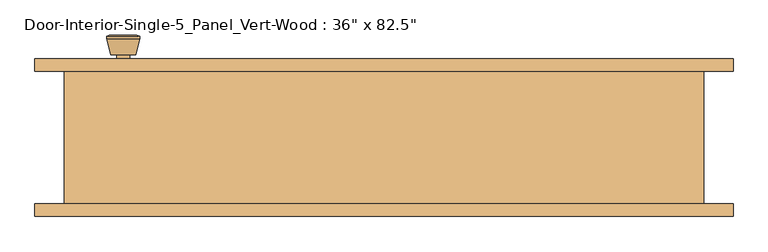
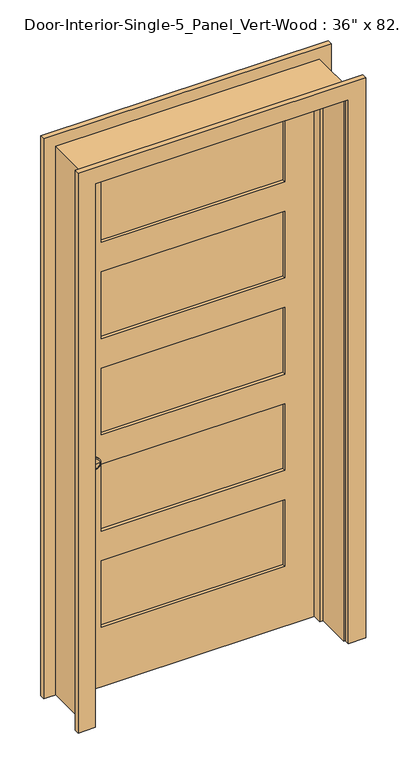
"""IFC4 building model written with IfcOpenShell, lengths in millimetres: door geometry."""

from ifc_helpers import new_model, si_unit, point, frame, frame_2d, origin, place, context, project, spatial, polyline, circle_curve, trimmed, segment, composite_curve, outline, extrude, faceted_brep, source, transform, mapped, element, save
from ifc_brep_helpers import plane_surface, cylinder_surface, revolved_surface, advanced_brep


def door_3f7a11fd(model_context):
    return source(origin(), model_context, "Body", "SolidModel", [
        advanced_brep(
        [(-393.7, 55.9, 914.4), (-383.7, 55.9, 914.4), (-403.7, 55.9, 914.4), (-373.2241324, 6.9, 914.4), (-393.7, 6.9, 914.4), (-414.1758676, 6.9, 914.4), (-368.7, 8.7278681, 914.4), (-418.7, 8.7278681, 914.4), (-368.7, 12.1915463, 914.4), (-418.7, 12.1915463, 914.4), (-375.063764, 36.9, 914.4), (-412.336236, 36.9, 914.4), (-383.7, 36.9, 914.4), (-403.7, 36.9, 914.4)],
        [
            (0, 1),
            (1, 2, circle_curve(frame((-393.7, 55.9, 914.4), z_axis=(0.0, 1.0, 0.0), x_axis=(-1.0, 0.0, 0.0)), 10.0)),
            (2, 0),
            (2, 1, circle_curve(frame((-393.7, 55.9, 914.4), z_axis=(0.0, 1.0, 0.0), x_axis=(-1.0, 0.0, 0.0)), 10.0)),
            (3, 4),
            (4, 5),
            (5, 3, circle_curve(frame((-393.7, 6.9, 914.4), z_axis=(0.0, -1.0, 0.0), x_axis=(-1.0, 0.0, 0.0)), 20.4758676)),
            (3, 5, circle_curve(frame((-393.7, 6.9, 914.4), z_axis=(0.0, -1.0, 0.0), x_axis=(-1.0, 0.0, 0.0)), 20.4758676)),
            (6, 3),
            (5, 7),
            (7, 6, circle_curve(frame((-393.7, 8.7278681, 914.4), z_axis=(0.0, -1.0, 0.0), x_axis=(-1.0, 0.0, 0.0)), 25.0)),
            (6, 7, circle_curve(frame((-393.7, 8.7278681, 914.4), z_axis=(0.0, -1.0, 0.0), x_axis=(-1.0, 0.0, 0.0)), 25.0)),
            (8, 6),
            (7, 9),
            (9, 8, circle_curve(frame((-393.7, 12.1915463, 914.4), z_axis=(0.0, -1.0, 0.0), x_axis=(-1.0, 0.0, 0.0)), 25.0)),
            (8, 9, circle_curve(frame((-393.7, 12.1915463, 914.4), z_axis=(0.0, -1.0, 0.0), x_axis=(-1.0, 0.0, 0.0)), 25.0)),
            (10, 8),
            (9, 11),
            (11, 10, circle_curve(frame((-393.7, 36.9, 914.4), z_axis=(0.0, -1.0, 0.0), x_axis=(-1.0, 0.0, 0.0)), 18.636236)),
            (10, 11, circle_curve(frame((-393.7, 36.9, 914.4), z_axis=(0.0, -1.0, 0.0), x_axis=(-1.0, 0.0, 0.0)), 18.636236)),
            (12, 10),
            (11, 13),
            (13, 12, circle_curve(frame((-393.7, 36.9, 914.4), z_axis=(0.0, -1.0, 0.0), x_axis=(-1.0, 0.0, 0.0)), 10.0)),
            (12, 13, circle_curve(frame((-393.7, 36.9, 914.4), z_axis=(0.0, -1.0, 0.0), x_axis=(-1.0, 0.0, 0.0)), 10.0)),
            (1, 12),
            (13, 2),
        ],
        [
            plane_surface(frame((-393.7, 55.9, 914.4), z_axis=(0.0, 1.0, 0.0), x_axis=(-1.0, 0.0, 0.0))),
            plane_surface(frame((-393.7, 6.9, 914.4), z_axis=(0.0, -1.0, 0.0), x_axis=(-1.0, 0.0, 0.0))),
            revolved_surface(polyline([(-414.1758676, 6.9, 914.4), (-418.7, 8.7278681, 914.4)]), (-393.7, 55.9, 914.4), (0.0, 1.0, 0.0)),
            cylinder_surface(frame((-393.7, 55.9, 914.4), z_axis=(0.0, 1.0, 0.0), x_axis=(-1.0, 0.0, 0.0)), 25.0),
            revolved_surface(polyline([(-418.7, 12.1915463, 914.4), (-412.336236, 36.9, 914.4)]), (-393.7, 55.9, 914.4), (0.0, 1.0, 0.0)),
            plane_surface(frame((-393.7, 36.9, 914.4), z_axis=(0.0, 1.0, 0.0), x_axis=(-1.0, 0.0, 0.0))),
            cylinder_surface(frame((-393.7, 55.9, 914.4), z_axis=(0.0, 1.0, 0.0), x_axis=(-1.0, 0.0, 0.0)), 10.0),
        ],
        [
            (0, [[1, 2, 3]]),
            (0, [[-3, 4, -1]]),
            (1, [[5, 6, 7]]),
            (1, [[-6, -5, 8]]),
            (2, [[9, -7, 10, 11]]),
            (2, [[-10, -8, -9, 12]]),
            (3, [[13, -11, 14, 15]]),
            (3, [[-14, -12, -13, 16]]),
            (4, [[17, -15, 18, 19]]),
            (4, [[-18, -16, -17, 20]]),
            (5, [[21, -19, 22, 23]]),
            (5, [[-22, -20, -21, 24]]),
            (6, [[25, -23, 26, -2]]),
            (6, [[-26, -24, -25, -4]]),
        ],
    ),
        extrude(outline(composite_curve([segment(trimmed(circle_curve(frame_2d((914.4, -393.7)), 30.0), [point((914.4, -423.7))], [point((914.4, -363.7))], False, "CARTESIAN"), True, "CONTINUOUS"), segment(trimmed(circle_curve(frame_2d((914.4, -393.7)), 30.0), [point((914.4, -363.7))], [point((914.4, -423.7))], False, "CARTESIAN"), True, "CONTINUOUS")], self_intersect=False)), frame((0.0, 55.9, 0.0), z_axis=(0.0, 1.0, 0.0), x_axis=(0.0, 0.0, 1.0)), (0.0, 0.0, 1.0), 6.0),
        advanced_brep(
        [(-393.7, 102.825, 914.4), (-403.7, 102.825, 914.4), (-383.7, 102.825, 914.4), (-373.2241324, 151.825, 914.4), (-414.1758676, 151.825, 914.4), (-393.7, 151.825, 914.4), (-368.7, 149.9971319, 914.4), (-418.7, 149.9971319, 914.4), (-368.7, 146.5334537, 914.4), (-418.7, 146.5334537, 914.4), (-375.063764, 121.825, 914.4), (-412.336236, 121.825, 914.4), (-383.7, 121.825, 914.4), (-403.7, 121.825, 914.4)],
        [
            (0, 1),
            (1, 2, circle_curve(frame((-393.7, 102.825, 914.4), z_axis=(0.0, -1.0, 0.0), x_axis=(-1.0, 0.0, 0.0)), 10.0)),
            (2, 0),
            (2, 1, circle_curve(frame((-393.7, 102.825, 914.4), z_axis=(0.0, -1.0, 0.0), x_axis=(-1.0, 0.0, 0.0)), 10.0)),
            (3, 4, circle_curve(frame((-393.7, 151.825, 914.4), z_axis=(0.0, 1.0, 0.0), x_axis=(-1.0, 0.0, 0.0)), 20.4758676)),
            (4, 5),
            (5, 3),
            (4, 3, circle_curve(frame((-393.7, 151.825, 914.4), z_axis=(0.0, 1.0, 0.0), x_axis=(-1.0, 0.0, 0.0)), 20.4758676)),
            (6, 7, circle_curve(frame((-393.7, 149.9971319, 914.4), z_axis=(0.0, 1.0, 0.0), x_axis=(-1.0, 0.0, 0.0)), 25.0)),
            (7, 4),
            (3, 6),
            (7, 6, circle_curve(frame((-393.7, 149.9971319, 914.4), z_axis=(0.0, 1.0, 0.0), x_axis=(-1.0, 0.0, 0.0)), 25.0)),
            (8, 9, circle_curve(frame((-393.7, 146.5334537, 914.4), z_axis=(0.0, 1.0, 0.0), x_axis=(-1.0, 0.0, 0.0)), 25.0)),
            (9, 7),
            (6, 8),
            (9, 8, circle_curve(frame((-393.7, 146.5334537, 914.4), z_axis=(0.0, 1.0, 0.0), x_axis=(-1.0, 0.0, 0.0)), 25.0)),
            (10, 11, circle_curve(frame((-393.7, 121.825, 914.4), z_axis=(0.0, 1.0, 0.0), x_axis=(-1.0, 0.0, 0.0)), 18.636236)),
            (11, 9),
            (8, 10),
            (11, 10, circle_curve(frame((-393.7, 121.825, 914.4), z_axis=(0.0, 1.0, 0.0), x_axis=(-1.0, 0.0, 0.0)), 18.636236)),
            (12, 13, circle_curve(frame((-393.7, 121.825, 914.4), z_axis=(0.0, 1.0, 0.0), x_axis=(-1.0, 0.0, 0.0)), 10.0)),
            (13, 11),
            (10, 12),
            (13, 12, circle_curve(frame((-393.7, 121.825, 914.4), z_axis=(0.0, 1.0, 0.0), x_axis=(-1.0, 0.0, 0.0)), 10.0)),
            (1, 13),
            (12, 2),
        ],
        [
            plane_surface(frame((-393.7, 102.825, 914.4), z_axis=(0.0, -1.0, 0.0), x_axis=(-1.0, 0.0, 0.0))),
            plane_surface(frame((-393.7, 151.825, 914.4), z_axis=(0.0, 1.0, 0.0), x_axis=(-1.0, 0.0, 0.0))),
            revolved_surface(polyline([(-414.1758676, 151.825, 914.4), (-418.7, 149.9971319, 914.4)]), (-393.7, 102.825, 914.4), (0.0, -1.0, 0.0)),
            cylinder_surface(frame((-393.7, 102.825, 914.4), z_axis=(0.0, -1.0, 0.0), x_axis=(-1.0, 0.0, 0.0)), 25.0),
            revolved_surface(polyline([(-418.7, 146.5334537, 914.4), (-412.336236, 121.825, 914.4)]), (-393.7, 102.825, 914.4), (0.0, -1.0, 0.0)),
            plane_surface(frame((-393.7, 121.825, 914.4), z_axis=(0.0, -1.0, 0.0), x_axis=(-1.0, 0.0, 0.0))),
            cylinder_surface(frame((-393.7, 102.825, 914.4), z_axis=(0.0, -1.0, 0.0), x_axis=(-1.0, 0.0, 0.0)), 10.0),
        ],
        [
            (0, [[1, 2, 3]]),
            (0, [[-3, 4, -1]]),
            (1, [[5, 6, 7]]),
            (1, [[8, -7, -6]]),
            (2, [[9, 10, -5, 11]]),
            (2, [[12, -11, -8, -10]]),
            (3, [[13, 14, -9, 15]]),
            (3, [[16, -15, -12, -14]]),
            (4, [[17, 18, -13, 19]]),
            (4, [[20, -19, -16, -18]]),
            (5, [[21, 22, -17, 23]]),
            (5, [[24, -23, -20, -22]]),
            (6, [[-2, 25, -21, 26]]),
            (6, [[-4, -26, -24, -25]]),
        ],
    ),
        extrude(outline(composite_curve([segment(trimmed(circle_curve(frame_2d((914.4, -393.7)), 30.0), [point((914.4, -423.7))], [point((914.4, -363.7))], False, "CARTESIAN"), True, "CONTINUOUS"), segment(trimmed(circle_curve(frame_2d((914.4, -393.7)), 30.0), [point((914.4, -363.7))], [point((914.4, -423.7))], False, "CARTESIAN"), True, "CONTINUOUS")], self_intersect=False)), frame((0.0, 96.825, 0.0), z_axis=(0.0, 1.0, 0.0), x_axis=(0.0, 0.0, 1.0)), (0.0, 0.0, 1.0), 6.0),
        faceted_brep([(482.6, 96.825, 0.0), (482.6, -103.175, 0.0), (457.2, -103.175, 0.0), (457.2, 26.975, 0.0), (444.5, 26.975, 0.0), (444.5, 61.9, 0.0), (457.2, 61.9, 0.0), (457.2, 96.825, 0.0), (482.6, 96.825, 2125.4), (482.6, -103.175, 2125.4), (-482.6, -103.175, 2125.4), (-482.6, -103.175, 0.0), (-457.2, -103.175, 0.0), (-457.2, -103.175, 2100.0), (457.2, -103.175, 2100.0), (457.2, 26.975, 2100.0), (-457.2, 26.975, 2100.0), (-457.2, 26.975, 0.0), (-444.5, 26.975, 0.0), (-444.5, 26.975, 2087.3), (444.5, 26.975, 2087.3), (444.5, 61.9, 2087.3), (-444.5, 61.9, 2087.3), (-444.5, 61.9, 0.0), (-457.2, 61.9, 0.0), (-457.2, 61.9, 2100.0), (457.2, 61.9, 2100.0), (457.2, 96.825, 2100.0), (-457.2, 96.825, 2100.0), (-457.2, 96.825, 0.0), (-482.6, 96.825, 0.0), (-482.6, 96.825, 2125.4)], [[[0, 1, 2, 3, 4, 5, 6, 7]], [[1, 0, 8, 9]], [[2, 1, 9, 10, 11, 12, 13, 14]], [[3, 2, 14, 15]], [[4, 3, 15, 16, 17, 18, 19, 20]], [[5, 4, 20, 21]], [[6, 5, 21, 22, 23, 24, 25, 26]], [[7, 6, 26, 27]], [[0, 7, 27, 28, 29, 30, 31, 8]], [[9, 8, 31, 10]], [[15, 14, 13, 16]], [[21, 20, 19, 22]], [[27, 26, 25, 28]], [[30, 29, 24, 23, 18, 17, 12, 11]], [[10, 31, 30, 11]], [[16, 13, 12, 17]], [[22, 19, 18, 23]], [[28, 25, 24, 29]]]),
        extrude(outline(polyline([(2100.0, -457.2), (0.0, -457.2), (0.0, 457.2), (2100.0, 457.2), (2100.0, -457.2)]), holes=[polyline([(1980.9375, -336.55), (1980.9375, 336.55), (1722.545, 336.55), (1722.545, -336.55), (1980.9375, -336.55)]), polyline([(490.1675, -336.55), (490.1675, 336.55), (231.775, 336.55), (231.775, -336.55), (490.1675, -336.55)]), polyline([(1235.5525, -336.55), (1235.5525, 336.55), (977.16, 336.55), (977.16, -336.55), (1235.5525, -336.55)]), polyline([(1608.245, -336.55), (1608.245, 336.55), (1349.8525, 336.55), (1349.8525, -336.55), (1608.245, -336.55)]), polyline([(862.86, -336.55), (862.86, 336.55), (604.4675, 336.55), (604.4675, -336.55), (862.86, -336.55)])]), frame((0.0, 61.9, 0.0), z_axis=(0.0, 1.0, 0.0), x_axis=(0.0, 0.0, 1.0)), (0.0, 0.0, 1.0), 34.925),
        extrude(outline(polyline([(336.55, 73.5416667), (-336.55, 73.5416667), (-336.55, 85.1833333), (336.55, 85.1833333), (336.55, 73.5416667)])), frame((0.0, 0.0, 1722.545), z_axis=(0.0, 0.0, 1.0), x_axis=(1.0, 0.0, 0.0)), (0.0, 0.0, 1.0), 258.3925),
        extrude(outline(polyline([(336.55, 73.5416667), (-336.55, 73.5416667), (-336.55, 85.1833333), (336.55, 85.1833333), (336.55, 73.5416667)])), frame((0.0, 0.0, 1349.8525), z_axis=(0.0, 0.0, 1.0), x_axis=(1.0, 0.0, 0.0)), (0.0, 0.0, 1.0), 258.3925),
        extrude(outline(polyline([(336.55, 73.5416667), (-336.55, 73.5416667), (-336.55, 85.1833333), (336.55, 85.1833333), (336.55, 73.5416667)])), frame((0.0, 0.0, 604.4675), z_axis=(0.0, 0.0, 1.0), x_axis=(1.0, 0.0, 0.0)), (0.0, 0.0, 1.0), 258.3925),
        extrude(outline(polyline([(336.55, 73.5416667), (-336.55, 73.5416667), (-336.55, 85.1833333), (336.55, 85.1833333), (336.55, 73.5416667)])), frame((0.0, 0.0, 231.775), z_axis=(0.0, 0.0, 1.0), x_axis=(1.0, 0.0, 0.0)), (0.0, 0.0, 1.0), 258.3925),
        extrude(outline(polyline([(336.55, 73.5416667), (-336.55, 73.5416667), (-336.55, 85.1833333), (336.55, 85.1833333), (336.55, 73.5416667)])), frame((0.0, 0.0, 977.16), z_axis=(0.0, 0.0, 1.0), x_axis=(1.0, 0.0, 0.0)), (0.0, 0.0, 1.0), 258.3925),
        extrude(outline(polyline([(0.0, 463.55), (0.0, 527.05), (2169.85, 527.05), (2169.85, -527.05), (0.0, -527.05), (0.0, -463.55), (2106.35, -463.55), (2106.35, 463.55), (0.0, 463.55)])), frame((0.0, 96.825, 0.0), z_axis=(0.0, 1.0, 0.0), x_axis=(0.0, 0.0, 1.0)), (0.0, 0.0, 1.0), 19.05),
        extrude(outline(polyline([(0.0, 463.55), (0.0, 527.05), (2169.85, 527.05), (2169.85, -527.05), (0.0, -527.05), (0.0, -463.55), (2106.35, -463.55), (2106.35, 463.55), (0.0, 463.55)])), frame((0.0, -122.225, 0.0), z_axis=(0.0, 1.0, 0.0), x_axis=(0.0, 0.0, 1.0)), (0.0, 0.0, 1.0), 19.05),
    ])


if __name__ == "__main__":
    model = new_model("IFC4")
    model_context = context("Model", 3, world=origin())
    ifc_project = project(units=[si_unit("LENGTHUNIT", "METRE", prefix="MILLI")], contexts=[model_context])
    site = spatial("IfcSite", under=ifc_project)
    building = spatial("IfcBuilding", under=site)
    placement = place(None, origin())
    door_shape = door_3f7a11fd(model_context)
    element("IfcDoor", 1, ObjectType="Door-Interior-Single-5_Panel_Vert-Wood : 36\" x 82.5\"", at=placement, inside=building, context=model_context, shape_type="MappedRepresentation", body=[
        mapped(door_shape, transform((0.0, 0.0, 0.0), x_axis=(1.0, 0.0, 0.0), y_axis=(0.0, 1.0, 0.0), z_axis=(0.0, 0.0, 1.0))),
    ])
    save(model, "model.ifc")

# Revit data of these elements
# Type "Door-Interior-Single-5_Panel_Vert-Wood : 36\" x 82.5\""
#   Type Mark = "20"
#   Assembly Code = "C1020300"
#   Analytic Construction = "Wooden"
#   Top Rail = 0' - 4 11/16"
#   Thickness = 0' - 1 3/8"
#   Thermal Resistance (R) = 2.5876 (h·ft²·°F)/BTU
#   Swing Angle [instance default] = 90.00°
#   Stiles = 0' - 4 3/4"
#   Rough Width = 3' - 2"
#   Rough Height = 6' - 11.67717"
#   Intermediate Rail = 0' - 4 1/2"
#   Height = 6' - 10.67717"
#   Width = 3' - 0"
#   Heat Transfer Coefficient (U) = 0.3865 BTU/(h·ft²·°F)
#   Bottom Rail = 0' - 9 1/8"
#   Trim Material = Cherry
#   Panel Material = Cherry
#   Frame Material = Cherry
#   Door Handle Material = Aluminum
#   Visual Light Transmittance = 0
#   Solar Heat Gain Coefficient = 0
#   Wall Closure = (empty or 0)
#   Function = (empty or 0)
# Element 1 (IfcDoor, "Door-Interior-Single-5_Panel_Vert-Wood : 36\" x 82.5\"")
#   Materials on its faces: "Cherry", "Aluminum"
# Materials
#   "Cherry": class "Wood", colour RGB 226 177 128, transparency 0, Description = "Prunus Serotina", Cost = 0
#   "Aluminum": class "Metal", colour RGB 247 247 247, transparency 0, Description = "Aluminum 6061", Cost = 0
